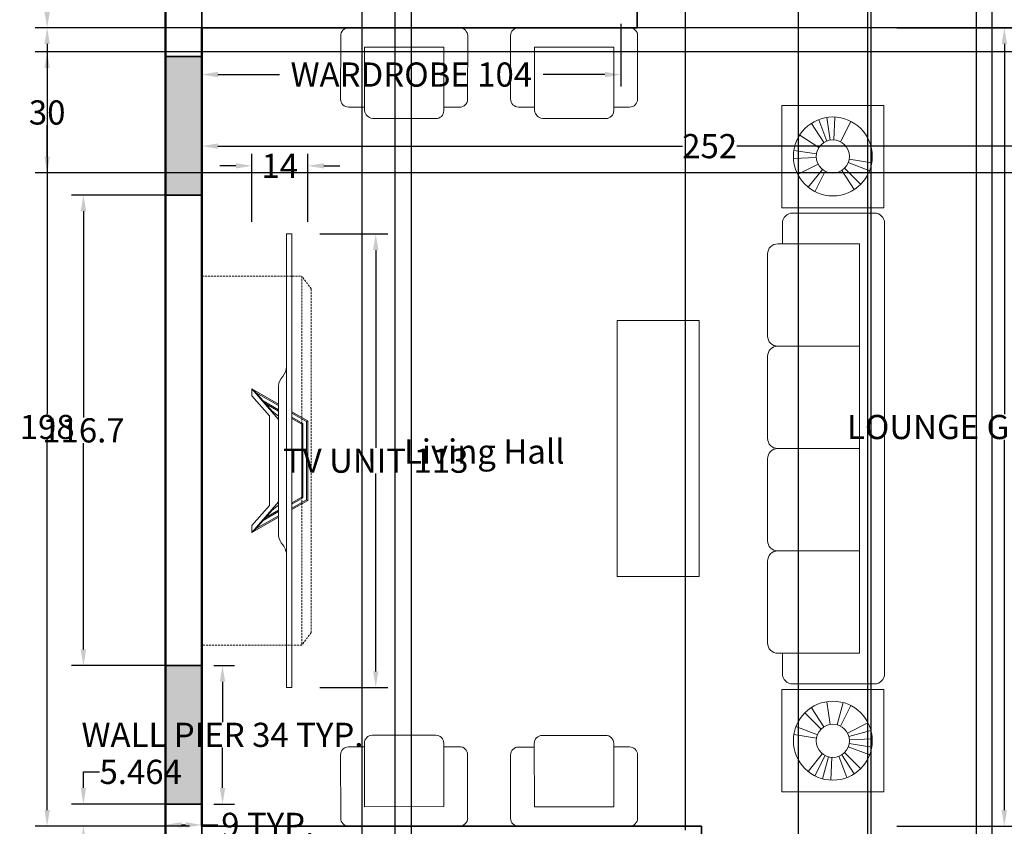
# Model space of a CAD drawing. Units: inches. Extents: x -1285 to -837, y -84 to 552.
# Tile 5 of 10: x -1282 to -1037, y 164 to 364. Entities that reach past the tile are written whole.
import ezdxf

# ---------------------------------------------------------------- set-up
doc = ezdxf.new("R2010")
doc.units = ezdxf.units.IN
doc.header["$MEASUREMENT"] = 0
doc.linetypes.add('DASHED', pattern=[0.75, 0.5, -0.25])
for name, color, linetype, lineweight in [('A-ANNO-DIMS', 2, 'Continuous', 18), ('A-AREA-IDEN', 7, 'Continuous', 25), ('A-COLS', 54, 'Continuous', 35), ('A-COLS-PATT', 54, 'Continuous', 13), ('A-FURN-CSWK', 9, 'Continuous', 18), ('A-FURN-CSWK-HIDN', 9, 'DASHED', 13), ('Inner Wall', 202, 'Continuous', 35), ('Outer Wall', 12, 'Continuous', 50), ('Sofa', 41, 'Continuous', 18), ('TV block', 50, 'Continuous', 18)]:
    doc.layers.add(name, color=color, linetype=linetype, lineweight=lineweight)
doc.styles.get("Standard").update_dxf_attribs({"font": 'arial.ttf'})
doc.dimstyles.get("Standard").update_dxf_attribs({"dimtxt": 6, "dimasz": 4, "dimexe": 3, "dimexo": 3, "dimgap": 0.09, "dimtad": 0, "dimtih": 1, "dimtoh": 1, "dimdec": 1, "dimzin": 0, "dimdsep": 46, "dimlunit": 3, "dimtxsty": 'Standard', "dimcen": 0.09, "dimadec": 0, "dimazin": 0, "dimtfac": 1, "dimtdec": 1, "dimtofl": 0, "dimtmove": 0, "dimatfit": 3, "dimfxl": 1, "dimtolj": 1, "dimtzin": 0, "dimarcsym": 0})

# ---------------------------------------------------------------- blocks, each defined once
blk = doc.blocks.new('TV Top view')
at = {"transparency": 33554687}
for points in [[(890.8, 1725.5), (939.4, 1640.4)], [(1299.3, 1640.4), (1348, 1725.5), (1250.7, 1640.4), (988, 1640.4), (890.8, 1725.5), (912.7, 1725.5), (976.4, 1669.8), (1262.3, 1669.8), (1326, 1725.5), (1348, 1725.5)], [(943.8, 1640.4), (902.7, 1712.3), (890.8, 1725.5)], [(902.7, 1712.3), (961.4, 1661), (977.5, 1640.4)], [(1336, 1712.3), (1277.3, 1661), (1261.2, 1640.4)], [(1348, 1725.5), (1336, 1712.3), (1294.9, 1640.4)], [(929, 1689.3), (956.9, 1640.4)], [(937.8, 1681.6), (961.3, 1640.4)], [(1300.9, 1681.6), (1277.4, 1640.4)], [(1309.7, 1689.3), (1281.8, 1640.4)], [(963.3, 1598.5), (992.4, 1547.7), (1246.4, 1547.7), (1275.4, 1598.5)], [(1271, 1598.5), (1244.1, 1551.5), (994.6, 1551.5), (967.7, 1598.5)], [(980.9, 1598.5), (1001.2, 1563), (1237.5, 1563), (1257.8, 1598.5)], [(1253.4, 1598.5), (1235.3, 1566.8), (1003.4, 1566.8), (985.3, 1598.5)], [(992.4, 1547.7), (994.6, 1551.5)], [(1001.2, 1563), (1003.4, 1566.8)], [(1237.5, 1563), (1235.3, 1566.8)], [(1246.4, 1547.7), (1244.1, 1551.5)]]:
    blk.add_lwpolyline(points, dxfattribs=at)
blk.add_lwpolyline([(814.6, 1615, 0.154134), (851.4, 1626.8, -0.181086), (878.4, 1640.4), (1358.2, 1640.4, -0.204566), (1387.4, 1626.8, 0.133001), (1419.3, 1615.2)], format="xyb", dxfattribs=at)
blk.add_lwpolyline([(396.1, 1615), (1842.6, 1615), (1842.6, 1598.5), (396.1, 1598.5)], close=True, dxfattribs=at)
blk = doc.blocks.new('Sofa Set')
for p, q in [((1019.14, 1064.07), (991.57, 1064.09)), ((1061.3, 1064.09), (1033.74, 1064.1)), ((989.59, 1046.4), (989.6, 1062.12)), ((1021.1, 1046.37), (1021.11, 1062.1)), ((1031.75, 1046.41), (1031.77, 1062.14)), ((1063.26, 1046.39), (1063.27, 1062.12)), ((995.51, 1059.29), (995.5, 1043.53)), ((995.51, 1059.29), (995.5, 1043.53)), ((995.51, 1059.29), (1015.2, 1059.27)), ((1015.19, 1043.52), (1015.2, 1059.27)), ((1037.67, 1059.31), (1037.66, 1043.55)), ((1037.67, 1059.31), (1037.66, 1043.55)), ((1037.67, 1059.31), (1057.36, 1059.29)), ((1057.35, 1043.54), (1057.36, 1059.29)), ((991.56, 1044.43), (995.5, 1044.42)), ((1019.13, 1044.41), (1015.19, 1044.41)), ((1033.72, 1044.44), (1037.66, 1044.44)), ((1061.29, 1044.43), (1057.35, 1044.43)), ((1099.01, 1044.85), (1124.39, 1044.85)), ((1099.01, 1019.47), (1099.01, 1044.85)), ((1124.39, 1044.85), (1124.39, 1019.47)), ((997.47, 1041.56), (1013.22, 1041.55)), ((1039.63, 1041.58), (1055.38, 1041.57)), ((1110.22, 1036), (1108.19, 1041.3)), ((1111.06, 1036.22), (1110.17, 1041.83)), ((1111.91, 1036.27), (1112.21, 1041.94)), ((1113.56, 1035.82), (1116.14, 1040.88)), ((1109.46, 1035.61), (1106.37, 1040.37)), ((1108.25, 1034.4), (1103.49, 1037.49)), ((1107.64, 1032.8), (1102.03, 1033.69)), ((1107.59, 1031.94), (1101.92, 1031.65)), ((1115.76, 1031.47), (1121.37, 1030.59)), ((1108.03, 1030.29), (1102.97, 1027.71)), ((1109.11, 1028.96), (1105.54, 1024.55)), ((1109.83, 1028.5), (1107.25, 1023.44)), ((1113.94, 1028.71), (1117.03, 1023.95)), ((1114.61, 1029.25), (1118.62, 1025.24)), ((1115.54, 1030.69), (1120.84, 1028.65)), ((1124.39, 1019.47), (1099.01, 1019.47)), ((1101.73, 1018.13), (1122, 1018.13)), ((1099.19, 1015.59), (1099.19, 1010.51)), ((1124.54, 903.9), (1124.54, 1015.59)), ((1098.04, 1010.51), (1118.35, 1010.51)), ((1118.35, 1010.51), (1118.35, 908.97)), ((1095.5, 987.66), (1095.5, 1007.97)), ((1098.04, 985.13), (1118.35, 985.13)), ((1095.5, 962.28), (1095.5, 982.59)), ((1098.04, 959.74), (1118.35, 959.74)), ((1095.5, 936.9), (1095.5, 957.2)), ((1118.35, 934.36), (1098.04, 934.36)), ((1118.35, 934.36), (1098.04, 934.36)), ((1095.5, 931.82), (1095.5, 911.51)), ((1098.04, 908.97), (1118.35, 908.97)), ((1099.19, 903.9), (1099.19, 908.97)), ((1101.73, 901.36), (1122, 901.36)), ((1099.01, 899.94), (1099.01, 874.56)), ((1124.39, 899.94), (1099.01, 899.94)), ((1124.39, 874.56), (1124.39, 899.94)), ((1111.06, 891.31), (1110.17, 896.92)), ((1112.76, 891.22), (1114.23, 896.71)), ((1108.79, 890.16), (1104.78, 894.18)), ((1109.46, 890.7), (1106.37, 895.46)), ((1113.56, 890.92), (1116.14, 895.98)), ((1115.36, 889.12), (1120.42, 891.7)), ((1107.86, 888.73), (1102.56, 890.76)), ((1115.67, 888.3), (1121.16, 889.77)), ((997.45, 888.61), (1013.2, 888.64)), ((1039.61, 888.57), (1055.36, 888.6)), ((1107.64, 887.9), (1102.03, 888.78)), ((1115.8, 887.45), (1121.48, 887.75)), ((991.55, 885.74), (995.48, 885.75)), ((995.51, 870.89), (995.48, 886.64)), ((995.51, 870.89), (995.48, 886.64)), ((1015.17, 886.67), (1015.19, 870.92)), ((1019.11, 885.79), (1015.17, 885.78)), ((1033.71, 885.7), (1037.65, 885.71)), ((1037.67, 870.85), (1037.64, 886.6)), ((1037.67, 870.85), (1037.64, 886.6)), ((1057.33, 886.63), (1057.35, 870.88)), ((1061.27, 885.74), (1057.33, 885.74)), ((1114.61, 884.34), (1118.62, 880.33)), ((1115.54, 885.78), (1120.84, 883.74)), ((1115.76, 886.59), (1121.37, 885.7)), ((989.58, 883.77), (989.6, 868.05)), ((1021.08, 883.82), (1021.1, 868.1)), ((1031.74, 883.73), (1031.76, 868.01)), ((1063.24, 883.78), (1063.27, 868.06)), ((1109.11, 884.06), (1105.54, 879.64)), ((1109.83, 883.59), (1107.25, 878.53)), ((1110.63, 883.28), (1109.16, 877.8)), ((1111.48, 883.15), (1111.19, 877.47)), ((1113.17, 883.41), (1115.21, 878.11)), ((1113.94, 883.8), (1117.03, 879.04)), ((1099.01, 874.56), (1124.39, 874.56)), ((995.51, 870.89), (1015.19, 870.92)), ((1037.67, 870.85), (1057.35, 870.88)), ((1019.14, 866.13), (991.57, 866.09)), ((1061.3, 866.09), (1033.74, 866.04))]:
    blk.add_line(p, q)
for centre, radius in [((1111.7, 1032.19), 9.79), ((1111.7, 1032.16), 4.11), ((1111.7, 887.28), 9.79), ((1111.7, 887.25), 4.11)]:
    blk.add_circle(centre, radius)
for centre, radius, start, end in [((991.57, 1062.12), 1.97, 89.96, 179.96), ((1019.14, 1062.1), 1.97, 359.96, 89.96), ((1033.73, 1062.14), 1.97, 89.96, 179.96), ((1061.3, 1062.12), 1.97, 359.96, 89.96), ((991.56, 1046.39), 1.97, 179.96, 269.96), ((1019.13, 1046.37), 1.97, 269.96, 359.96), ((1033.72, 1046.41), 1.97, 179.96, 269.96), ((1061.29, 1046.39), 1.97, 269.96, 359.96), ((998.04, 1044.1), 2.6, 192.5769, 257.3431), ((1013.22, 1043.52), 1.97, 269.96, 359.96), ((1040.2, 1044.12), 2.6, 192.5769, 257.3431), ((1055.38, 1043.54), 1.97, 269.96, 359.96), ((1101.73, 1015.59), 2.54, 90, 180), ((1122, 1015.59), 2.54, 0, 90), ((1098.04, 1007.97), 2.54, 90, 180), ((1098.04, 987.66), 2.54, 180, 270), ((1098.04, 982.59), 2.54, 90, 180), ((1098.04, 962.28), 2.54, 180, 270), ((1098.04, 957.2), 2.54, 90, 180), ((1098.04, 936.9), 2.54, 180, 270), ((1098.04, 931.82), 2.54, 90, 180), ((1098.04, 911.51), 2.54, 180, 270), ((1101.73, 903.9), 2.54, 180, 270), ((1122, 903.9), 2.54, 270, 0), ((997.45, 886.65), 1.97, 90.0848, 180.0848), ((1013.2, 886.67), 1.97, 0.0848, 90.0848), ((1039.61, 886.6), 1.97, 90.0848, 180.0848), ((1055.36, 886.63), 1.97, 0.0848, 90.0848), ((991.55, 883.78), 1.97, 90.0848, 180.0848), ((1019.11, 883.82), 1.97, 0.0848, 90.0848), ((1033.71, 883.74), 1.97, 90.0848, 180.0848), ((1061.27, 883.78), 1.97, 0.0848, 90.0848), ((991.57, 868.05), 1.97, 180.0848, 270.0848), ((1019.14, 868.09), 1.97, 270.0848, 0.0848), ((1033.73, 868.01), 1.97, 180.0848, 270.0848), ((1061.3, 868.05), 1.97, 270.0848, 0.0848)]:
    blk.add_arc(centre, radius, start, end)
blk = doc.blocks.new('WALL-PIER-34x9')
blk.add_lwpolyline([(9, 34.35), (9, 0), (0, 0), (0, 34.35)], close=True)
blk = doc.blocks.new('*D33')
at = {"layer": 'A-ANNO-DIMS', "color": 0, "lineweight": -2, "transparency": 16777216}
for p, q in [((-1233.53, 203.75), (-1228.38, 203.75)), ((-1231.38, 199.75), (-1231.38, 189.73)), ((-1231.38, 173.4), (-1231.38, 183.42)), ((-1233.53, 169.4), (-1228.38, 169.4))]:
    blk.add_line(p, q, dxfattribs=at)
at = {"layer": 'A-ANNO-DIMS', "color": 0, "transparency": 16777216}
for points in [[(-1232.04, 199.75), (-1230.71, 199.75), (-1231.38, 203.75)], [(-1232.04, 173.4), (-1230.71, 173.4), (-1231.38, 169.4)]]:
    blk.add_solid(points, dxfattribs=at)
at = {"layer": 'Defpoints', "color": 0, "transparency": 16777216}
for p in [(-1236.53, 203.75), (-1231.38, 203.75), (-1236.53, 169.4)]:
    blk.add_point(p, dxfattribs=at)
at = {"layer": 'A-ANNO-DIMS', "color": 0, "transparency": 16777216, "insert": (-1231.38, 186.58), "char_height": 6, "attachment_point": 5}
blk.add_mtext('\\A1;WALL PIER 34 TYP.', dxfattribs=at)
blk = doc.blocks.new('*D34')
at = {"layer": 'A-ANNO-DIMS', "color": 0, "lineweight": -2, "transparency": 16777216}
for p, q in [((-1245.53, 166.4), (-1245.53, 161.25)), ((-1236.53, 166.4), (-1236.53, 161.25)), ((-1241.53, 164.25), (-1240.53, 164.25)), ((-1236.53, 164.25), (-1232.53, 164.25))]:
    blk.add_line(p, q, dxfattribs=at)
at = {"layer": 'A-ANNO-DIMS', "color": 0, "transparency": 16777216}
for points in [[(-1241.53, 164.92), (-1241.53, 163.58), (-1245.53, 164.25)], [(-1240.53, 164.92), (-1240.53, 163.58), (-1236.53, 164.25)]]:
    blk.add_solid(points, dxfattribs=at)
at = {"layer": 'Defpoints', "color": 0, "transparency": 16777216}
for p in [(-1245.53, 169.4), (-1236.53, 169.4), (-1236.53, 164.25)]:
    blk.add_point(p, dxfattribs=at)
at = {"layer": 'A-ANNO-DIMS', "color": 0, "transparency": 16777216, "insert": (-1220.17, 164.25), "char_height": 6, "attachment_point": 5}
blk.add_mtext('\\A1;9 TYP.', dxfattribs=at)
blk = doc.blocks.new('*D55')
at = {"layer": 'A-ANNO-DIMS', "color": 0, "lineweight": -2, "transparency": 16777216}
for p, q in [((-1207.24, 310.83), (-1190.37, 310.83)), ((-1193.37, 306.83), (-1193.37, 257.73)), ((-1193.37, 202.32), (-1193.37, 251.42)), ((-1207.24, 198.32), (-1190.37, 198.32))]:
    blk.add_line(p, q, dxfattribs=at)
at = {"layer": 'A-ANNO-DIMS', "color": 0, "transparency": 16777216}
for points in [[(-1194.03, 306.83), (-1192.7, 306.83), (-1193.37, 310.83)], [(-1194.03, 202.32), (-1192.7, 202.32), (-1193.37, 198.32)]]:
    blk.add_solid(points, dxfattribs=at)
at = {"layer": 'Defpoints', "color": 0, "transparency": 16777216}
for p in [(-1210.24, 310.83), (-1193.37, 310.83), (-1210.24, 198.32)]:
    blk.add_point(p, dxfattribs=at)
at = {"layer": 'A-ANNO-DIMS', "color": 0, "transparency": 16777216, "insert": (-1193.37, 254.58), "char_height": 6, "attachment_point": 5}
blk.add_mtext('\\A1;TV UNIT 113', dxfattribs=at)
blk = doc.blocks.new('*D56')
at = {"layer": 'A-ANNO-DIMS', "color": 0, "lineweight": -2, "transparency": 16777216}
for p, q in [((-1224.07, 313.83), (-1224.07, 330.71)), ((-1210.24, 313.83), (-1210.24, 330.71)), ((-1228.07, 327.71), (-1232.07, 327.71)), ((-1206.24, 327.71), (-1202.24, 327.71))]:
    blk.add_line(p, q, dxfattribs=at)
at = {"layer": 'A-ANNO-DIMS', "color": 0, "transparency": 16777216}
for points in [[(-1228.07, 328.37), (-1228.07, 327.04), (-1224.07, 327.71)], [(-1206.24, 328.37), (-1206.24, 327.04), (-1210.24, 327.71)]]:
    blk.add_solid(points, dxfattribs=at)
at = {"layer": 'Defpoints', "color": 0, "transparency": 16777216}
for p in [(-1224.07, 327.71), (-1224.07, 310.83), (-1210.24, 310.83)]:
    blk.add_point(p, dxfattribs=at)
at = {"layer": 'A-ANNO-DIMS', "color": 0, "transparency": 16777216, "insert": (-1217.16, 327.71), "char_height": 6, "attachment_point": 5}
blk.add_mtext('\\A1;14', dxfattribs=at)
blk = doc.blocks.new('*D59')
at = {"layer": 'A-ANNO-DIMS', "color": 0, "lineweight": -2, "transparency": 16777216}
for p, q in [((-1236.53, 362.94), (-1236.53, 347.34)), ((-1132.53, 362.94), (-1132.53, 347.34)), ((-1232.53, 350.34), (-1217.2, 350.34)), ((-1136.53, 350.34), (-1151.86, 350.34))]:
    blk.add_line(p, q, dxfattribs=at)
at = {"layer": 'A-ANNO-DIMS', "color": 0, "transparency": 16777216}
for points in [[(-1232.53, 351.01), (-1232.53, 349.67), (-1236.53, 350.34)], [(-1136.53, 351.01), (-1136.53, 349.67), (-1132.53, 350.34)]]:
    blk.add_solid(points, dxfattribs=at)
at = {"layer": 'Defpoints', "color": 0, "transparency": 16777216}
for p in [(-1236.53, 365.94), (-1132.53, 365.94), (-1132.53, 350.34)]:
    blk.add_point(p, dxfattribs=at)
at = {"layer": 'A-ANNO-DIMS', "color": 0, "transparency": 16777216, "insert": (-1184.53, 350.34), "char_height": 6, "attachment_point": 5}
blk.add_mtext('\\A1;WARDROBE 104', dxfattribs=at)
blk = doc.blocks.new('*D65')
at = {"layer": 'A-ANNO-DIMS', "color": 0, "lineweight": -2, "transparency": 16777216}
for p, q in [((-1064.13, 361.96), (-1034.42, 361.96)), ((-1037.42, 357.96), (-1037.42, 266.12)), ((-1037.42, 167.9), (-1037.42, 259.73)), ((-1064.13, 163.9), (-1034.42, 163.9))]:
    blk.add_line(p, q, dxfattribs=at)
at = {"layer": 'A-ANNO-DIMS', "color": 0, "transparency": 16777216}
for points in [[(-1038.09, 357.96), (-1036.75, 357.96), (-1037.42, 361.96)], [(-1038.09, 167.9), (-1036.75, 167.9), (-1037.42, 163.9)]]:
    blk.add_solid(points, dxfattribs=at)
at = {"layer": 'Defpoints', "color": 0, "transparency": 16777216}
for p in [(-1067.13, 361.96), (-1037.42, 361.96), (-1067.13, 163.9)]:
    blk.add_point(p, dxfattribs=at)
at = {"layer": 'A-ANNO-DIMS', "color": 0, "transparency": 16777216, "insert": (-1037.42, 262.93), "char_height": 6, "attachment_point": 5}
blk.add_mtext('\\A1;LOUNGE GROUP 198', dxfattribs=at)
blk = doc.blocks.new('*D75')
at = {"layer": 'A-ANNO-DIMS', "color": 0, "lineweight": -2, "transparency": 16777216}
for p, q in [((-1239.53, 361.94), (-1277.88, 361.94)), ((-1274.88, 357.94), (-1274.88, 266.09)), ((-1274.88, 167.94), (-1274.88, 259.79)), ((-1239.53, 163.94), (-1277.88, 163.94))]:
    blk.add_line(p, q, dxfattribs=at)
at = {"layer": 'A-ANNO-DIMS', "color": 0, "transparency": 16777216}
for points in [[(-1275.55, 357.94), (-1274.21, 357.94), (-1274.88, 361.94)], [(-1275.55, 167.94), (-1274.21, 167.94), (-1274.88, 163.94)]]:
    blk.add_solid(points, dxfattribs=at)
at = {"layer": 'Defpoints', "color": 0, "transparency": 16777216}
for p in [(-1274.88, 361.94), (-1236.53, 361.94), (-1236.53, 163.94)]:
    blk.add_point(p, dxfattribs=at)
at = {"layer": 'A-ANNO-DIMS', "color": 0, "transparency": 16777216, "insert": (-1274.88, 262.94), "char_height": 6, "attachment_point": 5}
blk.add_mtext('\\A1;198', dxfattribs=at)
blk = doc.blocks.new('*D78')
at = {"layer": 'A-ANNO-DIMS', "color": 0, "lineweight": -2, "transparency": 16777216}
for p, q in [((-1236.53, 162.94), (-1236.53, 551.29)), ((-1116.53, 162.94), (-1116.53, 551.29)), ((-1232.53, 548.29), (-1182.96, 548.29)), ((-1120.53, 548.29), (-1170.1, 548.29))]:
    blk.add_line(p, q, dxfattribs=at)
at = {"layer": 'A-ANNO-DIMS', "color": 0, "transparency": 16777216}
for points in [[(-1232.53, 548.96), (-1232.53, 547.62), (-1236.53, 548.29)], [(-1120.53, 548.96), (-1120.53, 547.62), (-1116.53, 548.29)]]:
    blk.add_solid(points, dxfattribs=at)
at = {"layer": 'Defpoints', "color": 0, "transparency": 16777216}
for p in [(-1116.53, 548.29), (-1236.53, 159.94), (-1116.53, 159.94)]:
    blk.add_point(p, dxfattribs=at)
at = {"layer": 'A-ANNO-DIMS', "color": 0, "transparency": 16777216, "insert": (-1176.53, 548.29), "char_height": 6, "attachment_point": 5}
blk.add_mtext('\\A1;120', dxfattribs=at)
blk = doc.blocks.new('*D79')
at = {"layer": 'A-ANNO-DIMS', "color": 0, "lineweight": -2, "transparency": 16777216}
for p, q in [((-1236.53, 38.94), (-1236.53, 551.29)), ((-1188.53, 38.94), (-1188.53, 551.29)), ((-1232.53, 548.29), (-1217.04, 548.29)), ((-1192.53, 548.29), (-1208.02, 548.29))]:
    blk.add_line(p, q, dxfattribs=at)
at = {"layer": 'A-ANNO-DIMS', "color": 0, "transparency": 16777216}
for points in [[(-1232.53, 548.96), (-1232.53, 547.62), (-1236.53, 548.29)], [(-1192.53, 548.96), (-1192.53, 547.62), (-1188.53, 548.29)]]:
    blk.add_solid(points, dxfattribs=at)
at = {"layer": 'Defpoints', "color": 0, "transparency": 16777216}
for p in [(-1188.53, 548.29), (-1236.53, 35.94), (-1188.53, 35.94)]:
    blk.add_point(p, dxfattribs=at)
at = {"layer": 'A-ANNO-DIMS', "color": 0, "transparency": 16777216, "insert": (-1212.53, 548.29), "char_height": 6, "attachment_point": 5}
blk.add_mtext('\\A1;48', dxfattribs=at)
blk = doc.blocks.new('*D80')
at = {"layer": 'A-ANNO-DIMS', "color": 0, "lineweight": -2, "transparency": 16777216}
for p, q in [((-1184.53, -13.66), (-1184.53, 551.29)), ((-1032.53, -13.66), (-1032.53, 551.29)), ((-1180.53, 548.29), (-1114.94, 548.29)), ((-1036.53, 548.29), (-1102.12, 548.29))]:
    blk.add_line(p, q, dxfattribs=at)
at = {"layer": 'A-ANNO-DIMS', "color": 0, "transparency": 16777216}
for points in [[(-1180.53, 548.96), (-1180.53, 547.62), (-1184.53, 548.29)], [(-1036.53, 548.96), (-1036.53, 547.62), (-1032.53, 548.29)]]:
    blk.add_solid(points, dxfattribs=at)
at = {"layer": 'Defpoints', "color": 0, "transparency": 16777216}
for p in [(-1032.53, 548.29), (-1184.53, -16.66), (-1032.53, -16.66)]:
    blk.add_point(p, dxfattribs=at)
at = {"layer": 'A-ANNO-DIMS', "color": 0, "transparency": 16777216, "insert": (-1108.53, 548.29), "char_height": 6, "attachment_point": 5}
blk.add_mtext('\\A1;152', dxfattribs=at)
blk = doc.blocks.new('*D87')
at = {"layer": 'A-ANNO-DIMS', "color": 0, "lineweight": -2, "transparency": 16777216}
for p, q in [((-1070.53, 424.94), (-1070.53, -83.53)), ((-1040.53, 424.94), (-1040.53, -83.53)), ((-1066.53, -80.53), (-1059.9, -80.53)), ((-1044.53, -80.53), (-1051.15, -80.53))]:
    blk.add_line(p, q, dxfattribs=at)
at = {"layer": 'A-ANNO-DIMS', "color": 0, "transparency": 16777216}
for points in [[(-1066.53, -79.86), (-1066.53, -81.2), (-1070.53, -80.53)], [(-1044.53, -79.86), (-1044.53, -81.2), (-1040.53, -80.53)]]:
    blk.add_solid(points, dxfattribs=at)
at = {"layer": 'Defpoints', "color": 0, "transparency": 16777216}
for p in [(-1070.53, 427.94), (-1040.53, 427.94), (-1040.53, -80.53)]:
    blk.add_point(p, dxfattribs=at)
at = {"layer": 'A-ANNO-DIMS', "color": 0, "transparency": 16777216, "insert": (-1055.53, -80.53), "char_height": 6, "attachment_point": 5}
blk.add_mtext('\\A1;30', dxfattribs=at)
blk = doc.blocks.new('*D88')
at = {"layer": 'A-ANNO-DIMS', "color": 0, "lineweight": -2, "transparency": 16777216}
for p, q in [((-987.53, 355.94), (-1277.88, 355.94)), ((-1274.88, 351.94), (-1274.88, 344.09)), ((-1274.88, 329.94), (-1274.88, 337.78)), ((-987.53, 325.94), (-1277.88, 325.94))]:
    blk.add_line(p, q, dxfattribs=at)
at = {"layer": 'A-ANNO-DIMS', "color": 0, "transparency": 16777216}
for points in [[(-1275.55, 351.94), (-1274.21, 351.94), (-1274.88, 355.94)], [(-1275.55, 329.94), (-1274.21, 329.94), (-1274.88, 325.94)]]:
    blk.add_solid(points, dxfattribs=at)
at = {"layer": 'Defpoints', "color": 0, "transparency": 16777216}
for p in [(-1274.88, 355.94), (-984.53, 355.94), (-984.53, 325.94)]:
    blk.add_point(p, dxfattribs=at)
at = {"layer": 'A-ANNO-DIMS', "color": 0, "transparency": 16777216, "insert": (-1274.88, 340.94), "char_height": 6, "attachment_point": 5}
blk.add_mtext('\\A1;30', dxfattribs=at)
blk = doc.blocks.new('*D96')
at = {"layer": 'A-ANNO-DIMS', "color": 0, "lineweight": -2, "transparency": 16777216}
for p, q in [((-1236.53, 506.94), (-1236.53, -83.53)), ((-1196.84, 506.94), (-1196.84, -83.53)), ((-1232.53, -80.53), (-1226.9, -80.53)), ((-1200.84, -80.53), (-1206.47, -80.53))]:
    blk.add_line(p, q, dxfattribs=at)
at = {"layer": 'A-ANNO-DIMS', "color": 0, "transparency": 16777216}
for points in [[(-1232.53, -79.86), (-1232.53, -81.2), (-1236.53, -80.53)], [(-1200.84, -79.86), (-1200.84, -81.2), (-1196.84, -80.53)]]:
    blk.add_solid(points, dxfattribs=at)
at = {"layer": 'Defpoints', "color": 0, "transparency": 16777216}
for p in [(-1236.53, 509.94), (-1196.84, 509.94), (-1196.84, -80.53)]:
    blk.add_point(p, dxfattribs=at)
at = {"layer": 'A-ANNO-DIMS', "color": 0, "transparency": 16777216, "insert": (-1216.68, -80.53), "char_height": 6, "attachment_point": 5}
blk.add_mtext('\\A1;39.69', dxfattribs=at)
blk = doc.blocks.new('*D103')
at = {"layer": 'A-ANNO-DIMS', "color": 0, "lineweight": -2, "transparency": 16777216}
for p, q in [((-1088.53, 506.94), (-1088.53, -83.53)), ((-1071.35, 506.94), (-1071.35, -83.53)), ((-1084.53, -80.53), (-1075.35, -80.53)), ((-1071.35, -80.53), (-1067.35, -80.53))]:
    blk.add_line(p, q, dxfattribs=at)
at = {"layer": 'A-ANNO-DIMS', "color": 0, "transparency": 16777216}
for points in [[(-1084.53, -79.86), (-1084.53, -81.2), (-1088.53, -80.53)], [(-1075.35, -79.86), (-1075.35, -81.2), (-1071.35, -80.53)]]:
    blk.add_solid(points, dxfattribs=at)
at = {"layer": 'Defpoints', "color": 0, "transparency": 16777216}
for p in [(-1088.53, 509.94), (-1071.35, 509.94), (-1071.35, -80.53)]:
    blk.add_point(p, dxfattribs=at)
at = {"layer": 'A-ANNO-DIMS', "color": 0, "transparency": 16777216, "insert": (-1057.41, -80.53), "char_height": 6, "attachment_point": 5}
blk.add_mtext('\\A1;17.18', dxfattribs=at)
blk = doc.blocks.new('*D104')
at = {"layer": 'A-ANNO-DIMS', "color": 0, "lineweight": -2, "transparency": 16777216}
for p, q in [((-1044.37, 506.94), (-1044.37, -83.53)), ((-1034.53, 506.94), (-1034.53, -83.53)), ((-1040.37, -80.53), (-1038.53, -80.53)), ((-1034.53, -80.53), (-1030.53, -80.53))]:
    blk.add_line(p, q, dxfattribs=at)
at = {"layer": 'A-ANNO-DIMS', "color": 0, "transparency": 16777216}
for points in [[(-1040.37, -79.86), (-1040.37, -81.2), (-1044.37, -80.53)], [(-1038.53, -79.86), (-1038.53, -81.2), (-1034.53, -80.53)]]:
    blk.add_solid(points, dxfattribs=at)
at = {"layer": 'Defpoints', "color": 0, "transparency": 16777216}
for p in [(-1044.37, 509.94), (-1034.53, 509.94), (-1034.53, -80.53)]:
    blk.add_point(p, dxfattribs=at)
at = {"layer": 'A-ANNO-DIMS', "color": 0, "transparency": 16777216, "insert": (-1022.66, -80.53), "char_height": 6, "attachment_point": 5}
blk.add_mtext('\\A1;9.84', dxfattribs=at)
blk = doc.blocks.new('*D105')
at = {"layer": 'A-ANNO-DIMS', "color": 0, "lineweight": -2, "transparency": 16777216}
for p, q in [((-1088.53, 428.94), (-1088.53, -83.53)), ((-1070.53, 428.94), (-1070.53, -83.53)), ((-1084.53, -80.53), (-1083.64, -80.53)), ((-1074.53, -80.53), (-1075.42, -80.53))]:
    blk.add_line(p, q, dxfattribs=at)
at = {"layer": 'A-ANNO-DIMS', "color": 0, "transparency": 16777216}
for points in [[(-1084.53, -79.86), (-1084.53, -81.2), (-1088.53, -80.53)], [(-1074.53, -79.86), (-1074.53, -81.2), (-1070.53, -80.53)]]:
    blk.add_solid(points, dxfattribs=at)
at = {"layer": 'Defpoints', "color": 0, "transparency": 16777216}
for p in [(-1088.53, 431.94), (-1070.53, 431.94), (-1070.53, -80.53)]:
    blk.add_point(p, dxfattribs=at)
at = {"layer": 'A-ANNO-DIMS', "color": 0, "transparency": 16777216, "insert": (-1079.53, -80.53), "char_height": 6, "attachment_point": 5}
blk.add_mtext('\\A1;18', dxfattribs=at)
blk = doc.blocks.new('*D106')
at = {"layer": 'A-ANNO-DIMS', "color": 0, "lineweight": -2, "transparency": 16777216}
for p, q in [((-1274.88, 365.94), (-1274.88, 369.94)), ((-1274.88, 369.94), (-1270.88, 369.94)), ((-983.53, 361.94), (-1277.88, 361.94)), ((-983.53, 355.94), (-1277.88, 355.94)), ((-1274.88, 351.94), (-1274.88, 347.94))]:
    blk.add_line(p, q, dxfattribs=at)
at = {"layer": 'A-ANNO-DIMS', "color": 0, "transparency": 16777216}
for points in [[(-1275.55, 365.94), (-1274.21, 365.94), (-1274.88, 361.94)], [(-1275.55, 351.94), (-1274.21, 351.94), (-1274.88, 355.94)]]:
    blk.add_solid(points, dxfattribs=at)
at = {"layer": 'Defpoints', "color": 0, "transparency": 16777216}
for p in [(-1274.88, 361.94), (-980.53, 361.94), (-980.53, 355.94)]:
    blk.add_point(p, dxfattribs=at)
at = {"layer": 'A-ANNO-DIMS', "color": 0, "transparency": 16777216, "insert": (-1268.81, 369.94), "char_height": 6, "attachment_point": 5}
blk.add_mtext('\\A1;6', dxfattribs=at)
blk = doc.blocks.new('*D112')
at = {"layer": 'A-ANNO-DIMS', "color": 0, "lineweight": -2, "transparency": 16777216}
for p, q in [((-1239.53, 320.45), (-1268.88, 320.45)), ((-1265.88, 316.45), (-1265.88, 265.25)), ((-1265.88, 207.75), (-1265.88, 258.95)), ((-1239.53, 203.75), (-1268.88, 203.75))]:
    blk.add_line(p, q, dxfattribs=at)
at = {"layer": 'A-ANNO-DIMS', "color": 0, "transparency": 16777216}
for points in [[(-1266.55, 316.45), (-1265.21, 316.45), (-1265.88, 320.45)], [(-1266.55, 207.75), (-1265.21, 207.75), (-1265.88, 203.75)]]:
    blk.add_solid(points, dxfattribs=at)
at = {"layer": 'Defpoints', "color": 0, "transparency": 16777216}
for p in [(-1265.88, 320.45), (-1236.53, 320.45), (-1236.53, 203.75)]:
    blk.add_point(p, dxfattribs=at)
at = {"layer": 'A-ANNO-DIMS', "color": 0, "transparency": 16777216, "insert": (-1265.88, 262.1), "char_height": 6, "attachment_point": 5}
blk.add_mtext('\\A1;116.7', dxfattribs=at)
blk = doc.blocks.new('*D113')
at = {"layer": 'A-ANNO-DIMS', "color": 0, "lineweight": -2, "transparency": 16777216}
for p, q in [((-1265.88, 173.4), (-1265.88, 177.4)), ((-1265.88, 177.4), (-1261.88, 177.4)), ((-1239.53, 169.4), (-1268.88, 169.4)), ((-1239.53, 163.94), (-1268.88, 163.94)), ((-1265.88, 159.94), (-1265.88, 155.94))]:
    blk.add_line(p, q, dxfattribs=at)
at = {"layer": 'A-ANNO-DIMS', "color": 0, "transparency": 16777216}
for points in [[(-1266.55, 173.4), (-1265.21, 173.4), (-1265.88, 169.4)], [(-1266.55, 159.94), (-1265.21, 159.94), (-1265.88, 163.94)]]:
    blk.add_solid(points, dxfattribs=at)
at = {"layer": 'Defpoints', "color": 0, "transparency": 16777216}
for p in [(-1265.88, 169.4), (-1236.53, 169.4), (-1236.53, 163.94)]:
    blk.add_point(p, dxfattribs=at)
at = {"layer": 'A-ANNO-DIMS', "color": 0, "transparency": 16777216, "insert": (-1251.68, 177.4), "char_height": 6, "attachment_point": 5}
blk.add_mtext('\\A1;5.464', dxfattribs=at)
blk = doc.blocks.new('*D119')
at = {"layer": 'A-ANNO-DIMS', "color": 0, "lineweight": -2, "transparency": 16777216}
for p, q in [((-1236.53, 358.94), (-1236.53, 329.59)), ((-984.53, 358.94), (-984.53, 329.59)), ((-1232.53, 332.59), (-1117.27, 332.59)), ((-988.53, 332.59), (-1103.79, 332.59))]:
    blk.add_line(p, q, dxfattribs=at)
at = {"layer": 'A-ANNO-DIMS', "color": 0, "transparency": 16777216}
for points in [[(-1232.53, 333.26), (-1232.53, 331.92), (-1236.53, 332.59)], [(-988.53, 333.26), (-988.53, 331.92), (-984.53, 332.59)]]:
    blk.add_solid(points, dxfattribs=at)
at = {"layer": 'Defpoints', "color": 0, "transparency": 16777216}
for p in [(-1236.53, 361.94), (-984.53, 361.94), (-1236.53, 332.59)]:
    blk.add_point(p, dxfattribs=at)
at = {"layer": 'A-ANNO-DIMS', "color": 0, "transparency": 16777216, "insert": (-1110.53, 332.59), "char_height": 6, "attachment_point": 5}
blk.add_mtext('\\A1;252', dxfattribs=at)

msp = doc.modelspace()

# ---------------------------------------------------------------- hatches: boundary and pattern name
at = {"layer": 'A-COLS-PATT'}
h = msp.add_hatch(color=256, dxfattribs=at)
h.dxf.hatch_style = 1
h.paths.add_polyline_path([(-1236.5299, 354.7957), (-1245.5299, 354.7957), (-1245.5299, 320.4471), (-1236.5299, 320.4471)])
h.paths.add_polyline_path([(-1236.5299, 466.4307), (-1245.5299, 466.4307), (-1245.5299, 432.0821), (-1236.5299, 432.0821)])
h.paths.add_polyline_path([(-877.5299, 151.7586), (-886.5299, 151.7586), (-886.5299, 117.41), (-877.5299, 117.41)])
h.paths.add_polyline_path([(-877.5299, 43.9103), (-886.5299, 43.9103), (-886.5299, -28.0897), (-877.5299, -28.0897)])
h.paths.add_polyline_path([(-1236.5299, 203.7523), (-1245.5299, 203.7523), (-1245.5299, 169.4036), (-1236.5299, 169.4036)])

# ---------------------------------------------------------------- linework, layer by layer
at = {"layer": 'A-FURN-CSWK'}
msp.add_line((-1236.5242, 208.8515), (-1236.5242, 300.3072), dxfattribs=at)
at = {"layer": 'A-FURN-CSWK-HIDN'}
for p, q in [((-1236.5242, 300.3072), (-1211.7243, 300.3072)), ((-1211.7243, 300.3072), (-1211.7243, 208.8515)), ((-1209.3563, 297.2072), (-1211.7243, 300.3072)), ((-1209.3563, 297.2072), (-1209.3563, 211.9497)), ((-1209.3563, 211.9497), (-1211.7243, 208.8515)), ((-1211.7243, 208.8515), (-1236.5299, 208.8515))]:
    msp.add_line(p, q, dxfattribs=at)
at = {"layer": 'Inner Wall'}
for p, q in [((-1128.5299, 371.9392), (-1128.5299, 361.9392)), ((-1236.5299, 361.9392), (-1128.5299, 361.9392)), ((-1236.5299, 163.9392), (-1112.5299, 163.9392)), ((-1112.5299, 163.9392), (-1112.5299, 153.9392))]:
    msp.add_line(p, q, dxfattribs=at)
at = {"layer": 'Outer Wall'}
for p, q in [((-1245.5299, 518.9392), (-1245.5299, -51.0608)), ((-1236.5299, 361.9392), (-1236.5299, 163.9392))]:
    msp.add_line(p, q, dxfattribs=at)
at = {"layer": 'Sofa'}
msp.add_lwpolyline([(-1133.4614, 225.868), (-1133.4614, 289.3237), (-1113.1558, 289.3237), (-1113.1558, 225.868)], close=True, dxfattribs=at)

# ---------------------------------------------------------------- block references
at = {"layer": 'A-COLS'}
for p in [(-1245.53, 320.4471), (-1245.53, 169.4036)]:
    msp.add_blockref('WALL-PIER-34x9', p, dxfattribs=at)
at = {"layer": 'Sofa'}
msp.add_blockref('Sofa Set', (-2191.666, -702.1458), dxfattribs=at)
at = {"layer": 'TV block', "xscale": 0.0777811110444261, "yscale": 0.0777811110444261, "zscale": 0.0777811110444261, "rotation": 90}
msp.add_blockref('TV Top view', (-1089.8593, 167.5146), dxfattribs=at)

# ---------------------------------------------------------------- texts
at = {"layer": 'A-AREA-IDEN', "insert": (-1200.8307, 259.8474), "char_height": 6, "attachment_point": 1}
msp.add_mtext_dynamic_manual_height_columns('\\pxqc;Living Hall', width=68.784729, gutter_width=1, heights=[0], dxfattribs=at)

# ---------------------------------------------------------------- dimensions: what is measured, and where the dimension line sits
at = {"layer": 'A-ANNO-DIMS'}
for base, p1, p2, override, picture, middle in [((-1116.5299, 548.2892), (-1236.5299, 159.9392), (-1116.5299, 159.9392), {"dimdec": 0, "dimlfac": 1, "dimrnd": 0, "dimzin": 0, "dimdsep": 46, "dimlunit": 2}, '*D78', (-1176.5299, 548.2892)), ((-1188.5299, 548.2892), (-1236.5299, 35.9392), (-1188.5299, 35.9392), {"dimdec": 0, "dimlfac": 1, "dimrnd": 0, "dimzin": 0, "dimdsep": 46, "dimlunit": 2}, '*D79', (-1212.5299, 548.2892)), ((-1032.5299, 548.2892), (-1184.5299, -16.6608), (-1032.5299, -16.6608), {"dimdec": 0, "dimlfac": 1, "dimrnd": 0, "dimzin": 0, "dimdsep": 46, "dimlunit": 2}, '*D80', (-1108.5299, 548.2892)), ((-1196.8396, -80.5308), (-1236.5299, 509.9392), (-1196.8396, 509.9392), {"dimdec": 2, "dimlfac": 1, "dimrnd": 0, "dimzin": 0, "dimdsep": 46, "dimlunit": 2}, '*D96', (-1216.6847, -80.5308)), ((-1071.3483, -80.5308), (-1088.5299, 509.9392), (-1071.3483, 509.9392), {"dimdec": 2, "dimlfac": 1, "dimrnd": 0, "dimzin": 0, "dimdsep": 46, "dimlunit": 2}, '*D103', (-1057.4111, -80.5308)), ((-1034.5299, -80.5308), (-1044.3703, 509.9392), (-1034.5299, 509.9392), {"dimdec": 2, "dimlfac": 1, "dimrnd": 0, "dimzin": 0, "dimdsep": 46, "dimlunit": 2}, '*D104', (-1022.6595, -80.5308)), ((-1070.5299, -80.5308), (-1088.5299, 431.9392), (-1070.5299, 431.9392), {"dimdec": 0, "dimlfac": 1, "dimrnd": 0, "dimzin": 0, "dimdsep": 46, "dimlunit": 2}, '*D105', (-1079.5299, -80.5308)), ((-1040.5299, -80.5308), (-1070.5299, 427.9392), (-1040.5299, 427.9392), {"dimdec": 0, "dimlfac": 1, "dimrnd": 0, "dimzin": 0, "dimdsep": 46, "dimlunit": 2}, '*D87', (-1055.5299, -80.5308))]:
    dim = msp.add_linear_dim(base=base, p1=p1, p2=p2, dimstyle='Standard', override=override, dxfattribs=at)
    dim.commit()
    dim.dimension.update_dxf_attribs({"geometry": picture, "text_midpoint": middle})
for base, p1, p2, angle, override, picture, middle in [((-1274.8799, 361.9392), (-980.5299, 355.9392), (-980.5299, 361.9392), 90, {"dimdec": 0, "dimlfac": 1, "dimrnd": 0, "dimzin": 0, "dimdsep": 46, "dimlunit": 2}, '*D106', (-1268.809, 369.9392)), ((-1274.8799, 361.9392), (-1236.5299, 163.9392), (-1236.5299, 361.9392), 90, {"dimdec": 0, "dimlfac": 1, "dimrnd": 0, "dimzin": 0, "dimdsep": 46, "dimlunit": 2}, '*D75', (-1274.8799, 262.9392)), ((-1236.5299, 332.5892), (-984.5299, 361.9392), (-1236.5299, 361.9392), 180, {"dimdec": 0, "dimlfac": 1, "dimrnd": 0, "dimzin": 0, "dimdsep": 46, "dimlunit": 2}, '*D119', (-1110.5299, 332.5892)), ((-1274.8799, 355.9392), (-984.5299, 325.9392), (-984.5299, 355.9392), 90, {"dimdec": 0, "dimlfac": 1, "dimrnd": 0, "dimzin": 0, "dimdsep": 46, "dimlunit": 2}, '*D88', (-1274.8799, 340.9392)), ((-1224.072, 327.7078), (-1210.2425, 310.8317), (-1224.072, 310.8317), 180, {"dimdec": 0, "dimlfac": 1, "dimrnd": 0, "dimzin": 0, "dimdsep": 46, "dimlunit": 2}, '*D56', (-1217.1573, 327.7078)), ((-1265.8799, 320.4471), (-1236.5299, 203.7523), (-1236.5299, 320.4471), 90, {"dimdec": 1, "dimlfac": 1, "dimrnd": 0, "dimzin": 0, "dimdsep": 46, "dimlunit": 2}, '*D112', (-1265.8799, 262.0997)), ((-1265.8799, 169.4036), (-1236.5299, 163.9392), (-1236.5299, 169.4036), 90, {"dimdec": 3, "dimlfac": 1, "dimrnd": 0, "dimzin": 0, "dimdsep": 46, "dimlunit": 2}, '*D113', (-1251.6787, 177.4036))]:
    dim = msp.add_linear_dim(base=base, p1=p1, p2=p2, angle=angle, dimstyle='Standard', override=override, dxfattribs=at)
    dim.commit()
    dim.dimension.update_dxf_attribs({"geometry": picture, "text_midpoint": middle})
for base, p1, p2, text, picture, middle in [((-1132.5299, 350.3392), (-1236.5299, 365.9392), (-1132.5299, 365.9392), 'WARDROBE <>', '*D59', (-1184.5299, 350.3392)), ((-1236.5299, 164.2514), (-1245.5299, 169.4036), (-1236.5299, 169.4036), '<> TYP.', '*D34', (-1220.1677, 164.2514))]:
    dim = msp.add_linear_dim(base=base, p1=p1, p2=p2, text=text, dimstyle='Standard', override={"dimdec": 0, "dimlfac": 1, "dimrnd": 0, "dimzin": 0, "dimdsep": 46, "dimlunit": 2}, dxfattribs=at)
    dim.commit()
    dim.dimension.update_dxf_attribs({"geometry": picture, "text_midpoint": middle})
for base, p1, p2, text, picture, middle in [((-1037.4189, 361.9592), (-1067.1282, 163.8976), (-1067.1282, 361.9592), 'LOUNGE GROUP <>', '*D65', (-1037.4189, 262.9284)), ((-1193.3665, 310.8317), (-1210.2425, 198.3244), (-1210.2425, 310.8317), 'TV UNIT <>', '*D55', (-1193.3665, 254.5781)), ((-1231.3776, 203.7523), (-1236.5299, 169.4036), (-1236.5299, 203.7523), 'WALL PIER <> TYP.', '*D33', (-1231.3776, 186.5779))]:
    dim = msp.add_linear_dim(base=base, p1=p1, p2=p2, angle=90, text=text, dimstyle='Standard', override={"dimdec": 0, "dimlfac": 1, "dimrnd": 0, "dimzin": 0, "dimdsep": 46, "dimlunit": 2}, dxfattribs=at)
    dim.commit()
    dim.dimension.update_dxf_attribs({"geometry": picture, "text_midpoint": middle})

doc.saveas('drawing.dxf')
